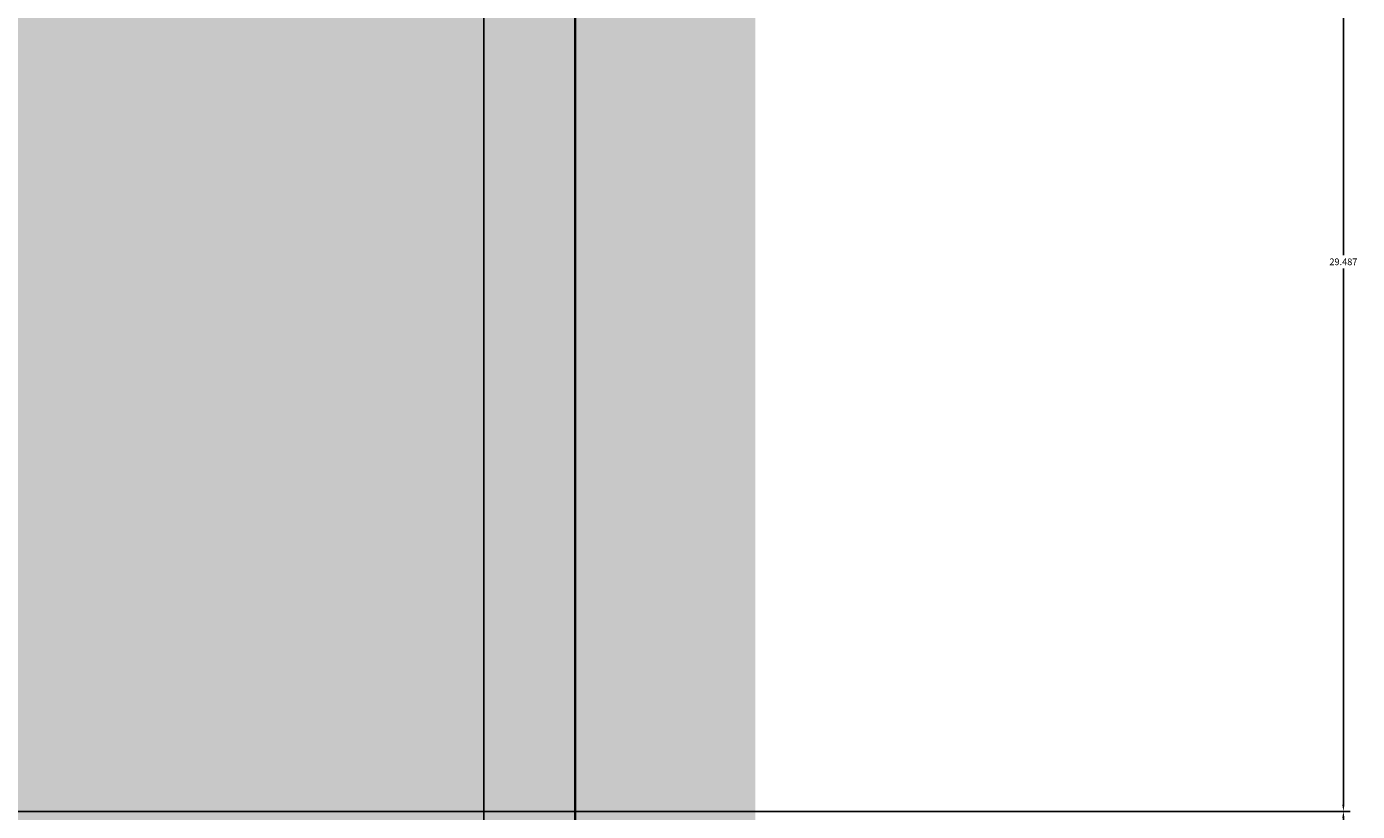
# Model space of a CAD drawing. Units: feet. Extents: x 2695 to 2912, y 795 to 1139.
# Tile 77 of 83: x 2876 to 2912, y 1021 to 1042. Entities that reach past the tile are written whole.
import ezdxf

# ---------------------------------------------------------------- set-up
doc = ezdxf.new("R2010")
doc.units = ezdxf.units.FT
for name, color, linetype, lineweight in [('A-ANNO-DIMS', 2, 'Continuous', 18), ('A-ELEV', 7, 'Continuous', 35), ('A-ELEV-PATT', 252, 'Continuous', 13)]:
    doc.layers.add(name, color=color, linetype=linetype, lineweight=lineweight)
doc.styles.get("Standard").update_dxf_attribs({"font": 'arial.ttf'})
doc.dimstyles.get("Standard").update_dxf_attribs({"dimtxt": 0.18, "dimasz": 0.18, "dimexe": 0.18, "dimexo": 0.0625, "dimgap": 0.09, "dimtad": 0, "dimtih": 1, "dimtoh": 1, "dimdec": 1, "dimzin": 0, "dimdsep": 46, "dimlunit": 3, "dimtxsty": 'Standard', "dimcen": 0.09, "dimadec": 0, "dimazin": 0, "dimtfac": 1, "dimtdec": 1, "dimtofl": 0, "dimtmove": 0, "dimatfit": 3, "dimfxl": 1, "dimtolj": 1, "dimtzin": 0, "dimarcsym": 0})

# ---------------------------------------------------------------- blocks, each defined once
blk = doc.blocks.new('*D11')
at = {"layer": 'A-ANNO-DIMS', "color": 0, "lineweight": -2, "transparency": 16777216}
for p, q in [((2843.575, 1020.886), (2843.575, 1138.886)), ((2843.755, 1138.706), (2869.128, 1138.706)), ((2895.289, 1138.706), (2869.916, 1138.706)), ((2895.469, 1107.898), (2895.469, 1138.886))]:
    blk.add_line(p, q, dxfattribs=at)
at = {"layer": 'A-ANNO-DIMS', "color": 0, "transparency": 16777216}
for points in [[(2843.755, 1138.736), (2843.755, 1138.676), (2843.575, 1138.706)], [(2895.289, 1138.736), (2895.289, 1138.676), (2895.469, 1138.706)]]:
    blk.add_solid(points, dxfattribs=at)
at = {"layer": 'Defpoints', "color": 0, "transparency": 16777216}
for p in [(2895.469, 1138.706), (2895.469, 1107.835), (2843.575, 1020.824)]:
    blk.add_point(p, dxfattribs=at)
at = {"layer": 'A-ANNO-DIMS', "color": 0, "transparency": 16777216, "insert": (2869.522, 1138.706), "char_height": 0.18, "attachment_point": 5}
blk.add_mtext('\\A1;51.89', dxfattribs=at)
blk = doc.blocks.new('*D17')
at = {"layer": 'A-ANNO-DIMS', "color": 0, "lineweight": -2, "transparency": 16777216}
for p, q in [((2843.637, 1020.824), (2911.424, 1020.824)), ((2911.244, 1020.644), (2911.244, 979.059)), ((2911.244, 937.111), (2911.244, 978.695)), ((2890.699, 936.931), (2911.424, 936.931))]:
    blk.add_line(p, q, dxfattribs=at)
at = {"layer": 'A-ANNO-DIMS', "color": 0, "transparency": 16777216}
for points in [[(2911.214, 1020.644), (2911.274, 1020.644), (2911.244, 1020.824)], [(2911.214, 937.111), (2911.274, 937.111), (2911.244, 936.931)]]:
    blk.add_solid(points, dxfattribs=at)
at = {"layer": 'Defpoints', "color": 0, "transparency": 16777216}
for p in [(2843.575, 1020.824), (2911.244, 1020.824), (2890.636, 936.931)]:
    blk.add_point(p, dxfattribs=at)
at = {"layer": 'A-ANNO-DIMS', "color": 0, "transparency": 16777216, "insert": (2911.244, 978.877), "char_height": 0.18, "attachment_point": 5}
blk.add_mtext('\\A1;83.9', dxfattribs=at)
blk = doc.blocks.new('*D18')
at = {"layer": 'A-ANNO-DIMS', "color": 0, "lineweight": -2, "transparency": 16777216}
for p, q in [((2890.699, 1050.311), (2911.424, 1050.311)), ((2911.244, 1050.131), (2911.244, 1035.749)), ((2911.244, 1021.004), (2911.244, 1035.385)), ((2843.637, 1020.824), (2911.424, 1020.824))]:
    blk.add_line(p, q, dxfattribs=at)
at = {"layer": 'A-ANNO-DIMS', "color": 0, "transparency": 16777216}
for points in [[(2911.214, 1050.131), (2911.274, 1050.131), (2911.244, 1050.311)], [(2911.214, 1021.004), (2911.274, 1021.004), (2911.244, 1020.824)]]:
    blk.add_solid(points, dxfattribs=at)
at = {"layer": 'Defpoints', "color": 0, "transparency": 16777216}
for p in [(2890.636, 1050.311), (2911.244, 1050.311), (2843.575, 1020.824)]:
    blk.add_point(p, dxfattribs=at)
at = {"layer": 'A-ANNO-DIMS', "color": 0, "transparency": 16777216, "insert": (2911.244, 1035.567), "char_height": 0.18, "attachment_point": 5}
blk.add_mtext('\\A1;29.487', dxfattribs=at)
blk = doc.blocks.new('*D50')
at = {"layer": 'A-ANNO-DIMS', "color": 0, "lineweight": -2, "transparency": 16777216}
for p, q in [((2810.041, 972.03), (2810.041, 1138.886)), ((2810.221, 1138.706), (2848.721, 1138.706)), ((2888.008, 1138.706), (2849.508, 1138.706)), ((2888.188, 972.03), (2888.188, 1138.886))]:
    blk.add_line(p, q, dxfattribs=at)
at = {"layer": 'A-ANNO-DIMS', "color": 0, "transparency": 16777216}
for points in [[(2810.221, 1138.736), (2810.221, 1138.676), (2810.041, 1138.706)], [(2888.008, 1138.736), (2888.008, 1138.676), (2888.188, 1138.706)]]:
    blk.add_solid(points, dxfattribs=at)
at = {"layer": 'Defpoints', "color": 0, "transparency": 16777216}
for p in [(2888.188, 1138.706), (2810.041, 971.967), (2888.188, 971.967)]:
    blk.add_point(p, dxfattribs=at)
at = {"layer": 'A-ANNO-DIMS', "color": 0, "transparency": 16777216, "insert": (2849.114, 1138.706), "char_height": 0.18, "attachment_point": 5}
blk.add_mtext('\\A1;78.15', dxfattribs=at)
blk = doc.blocks.new('*D51')
at = {"layer": 'A-ANNO-DIMS', "color": 0, "lineweight": -2, "transparency": 16777216}
for p, q in [((2888.188, 972.03), (2888.188, 1138.886)), ((2888.368, 1138.706), (2889.017, 1138.706)), ((2890.456, 1138.706), (2889.808, 1138.706)), ((2890.636, 972.03), (2890.636, 1138.886))]:
    blk.add_line(p, q, dxfattribs=at)
at = {"layer": 'A-ANNO-DIMS', "color": 0, "transparency": 16777216}
for points in [[(2888.368, 1138.736), (2888.368, 1138.676), (2888.188, 1138.706)], [(2890.456, 1138.736), (2890.456, 1138.676), (2890.636, 1138.706)]]:
    blk.add_solid(points, dxfattribs=at)
at = {"layer": 'Defpoints', "color": 0, "transparency": 16777216}
for p in [(2890.636, 1138.706), (2888.188, 971.967), (2890.636, 971.967)]:
    blk.add_point(p, dxfattribs=at)
at = {"layer": 'A-ANNO-DIMS', "color": 0, "transparency": 16777216, "insert": (2889.412, 1138.706), "char_height": 0.18, "attachment_point": 5}
blk.add_mtext('\\A1;2.448', dxfattribs=at)

msp = doc.modelspace()

# ---------------------------------------------------------------- hatches: boundary and pattern name
at = {"layer": 'A-ELEV-PATT'}
h = msp.add_hatch(color=256, dxfattribs=at)
h.set_gradient(color1=(147, 149, 152), color2=(147, 149, 152), tint=1)
h.paths.add_polyline_path([(2770.6361, 1118.4096), (2710.6361, 1118.4096), (2710.6361, 1062.9306), (2770.6361, 1062.9306)])
h.paths.add_polyline_path([(2890.6361, 1103.3378), (2770.6361, 1103.3378), (2770.6361, 1062.9306), (2890.6361, 1062.9306)])
h.paths.add_polyline_path([(2730.7081, 1048.1052), (2755.1125, 1048.1052), (2755.1125, 936.9306), (2770.6361, 936.9306), (2770.6361, 1050.3105), (2715.8852, 1050.3105), (2715.8852, 936.9306), (2730.7081, 936.9306)])
h.paths.add_polyline_path([(2890.6361, 1050.3105), (2770.6361, 1050.3105), (2770.6361, 971.9673), (2778.0341, 971.9673), (2778.0341, 1020.8235), (2843.575, 1020.8235), (2843.575, 971.9673), (2890.6361, 971.9673)])
h.paths.add_polyline_path([(2888.1882, 970.7156), (2843.575, 970.7156), (2843.575, 964.8267), (2888.1882, 964.8267)])
h.paths.add_polyline_path([(2888.1882, 964.1328), (2843.575, 964.1328), (2843.575, 956.614), (2888.1882, 956.614)])
h.paths.add_polyline_path([(2888.1882, 955.9202), (2843.575, 955.9202), (2843.575, 949.2892), (2888.1882, 949.2892)])
h.paths.add_polyline_path([(2888.1882, 948.5954), (2843.575, 948.5954), (2843.575, 941.3507), (2888.1882, 941.3507)])
h.paths.add_polyline_path([(2888.1882, 940.6569), (2843.575, 940.6569), (2843.575, 936.9306), (2888.1882, 936.9306)])
h.paths.add_polyline_path([(2890.6361, 970.7156), (2888.9368, 970.7156), (2888.9368, 964.8267), (2890.6361, 964.8267)])
h.paths.add_polyline_path([(2890.6361, 964.1328), (2888.9368, 964.1328), (2888.9368, 956.614), (2890.6361, 956.614)])
h.paths.add_polyline_path([(2890.6361, 955.9202), (2888.9368, 955.9202), (2888.9368, 949.2892), (2890.6361, 949.2892)])
h.paths.add_polyline_path([(2890.6361, 940.6569), (2888.9368, 940.6569), (2888.9368, 936.9306), (2890.6361, 936.9306)])
h.paths.add_polyline_path([(2890.6361, 948.5954), (2888.9368, 948.5954), (2888.9368, 941.3507), (2890.6361, 941.3507)])
h.paths.add_polyline_path([(2772.5216, 970.7156), (2770.6361, 970.7156), (2770.6361, 964.8267), (2772.5216, 964.8267)])
h.paths.add_polyline_path([(2772.5216, 964.1328), (2770.6361, 964.1328), (2770.6361, 956.614), (2772.5216, 956.614)])
h.paths.add_polyline_path([(2772.5216, 955.9202), (2770.6361, 955.9202), (2770.6361, 949.2892), (2772.5216, 949.2892)])
h.paths.add_polyline_path([(2772.5216, 948.5954), (2770.6361, 948.5954), (2770.6361, 941.3507), (2772.5216, 941.3507)])
h.paths.add_polyline_path([(2772.5216, 940.6569), (2770.6361, 940.6569), (2770.6361, 936.9306), (2772.5216, 936.9306)])
h.paths.add_polyline_path([(2778.0341, 940.6569), (2773.2702, 940.6569), (2773.2702, 936.9306), (2778.0341, 936.9306)])
h.paths.add_polyline_path([(2778.0341, 970.7156), (2773.2702, 970.7156), (2773.2702, 964.8267), (2778.0341, 964.8267)])
h.paths.add_polyline_path([(2778.0341, 964.1328), (2773.2702, 964.1328), (2773.2702, 956.614), (2778.0341, 956.614)])
h.paths.add_polyline_path([(2778.0341, 955.9202), (2773.2702, 955.9202), (2773.2702, 949.2892), (2778.0341, 949.2892)])
h.paths.add_polyline_path([(2778.0341, 948.5954), (2773.2702, 948.5954), (2773.2702, 941.3507), (2778.0341, 941.3507)])
h.paths.add_polyline_path([(2810.0407, 940.6569), (2780.0341, 940.6569), (2780.0341, 936.9306), (2810.0407, 936.9306)])
h.paths.add_polyline_path([(2890.6361, 924.3105), (2770.6361, 924.3105), (2770.6361, 810.9306), (2773.5029, 810.9306), (2773.5029, 905.5143), (2805.9398, 905.5143), (2838.3767, 905.5143), (2838.3767, 810.9306), (2890.6361, 810.9306)])
h = msp.add_hatch(color=256, dxfattribs=at)
h.set_gradient(color1=(255, 255, 255), tint=1)
h.paths.add_polyline_path([(2895.4694, 1107.8588), (2890.6361, 1107.8588), (2890.6361, 810.9306), (2895.4694, 810.9306)])
h = msp.add_hatch(color=256, dxfattribs=at)
h.set_gradient(color1=(255, 255, 255), tint=1)
h.paths.add_polyline_path([(2890.6361, 1050.3105), (2881.9484, 1050.3105), (2881.9484, 971.9673), (2890.6361, 971.9673)])
h.paths.add_polyline_path([(2888.1882, 970.7156), (2881.9484, 970.7156), (2881.9484, 964.8267), (2888.1882, 964.8267)])
h.paths.add_polyline_path([(2890.6361, 970.7156), (2888.9368, 970.7156), (2888.9368, 964.8267), (2890.6361, 964.8267)])
h.paths.add_polyline_path([(2888.1882, 964.1328), (2881.9484, 964.1328), (2881.9484, 956.614), (2888.1882, 956.614)])
h.paths.add_polyline_path([(2890.6361, 964.1328), (2888.9368, 964.1328), (2888.9368, 956.614), (2890.6361, 956.614)])
h.paths.add_polyline_path([(2888.1882, 955.9202), (2881.9484, 955.9202), (2881.9484, 949.2892), (2888.1882, 949.2892)])
h.paths.add_polyline_path([(2890.6361, 955.9202), (2888.9368, 955.9202), (2888.9368, 949.2892), (2890.6361, 949.2892)])
h.paths.add_polyline_path([(2888.1882, 948.5954), (2881.9484, 948.5954), (2881.9484, 941.3507), (2888.1882, 941.3507)])
h.paths.add_polyline_path([(2890.6361, 948.5954), (2888.9368, 948.5954), (2888.9368, 941.3507), (2890.6361, 941.3507)])
h.paths.add_polyline_path([(2888.1882, 940.6569), (2881.9484, 940.6569), (2881.9484, 936.9306), (2888.1882, 936.9306)])

# ---------------------------------------------------------------- linework, layer by layer
at = {"layer": 'A-ELEV'}
for p, q in [((2890.6361, 810.9306), (2890.6361, 1107.8588)), ((2890.6361, 1062.9306), (2890.6361, 810.9306))]:
    msp.add_line(p, q, dxfattribs=at)

# ---------------------------------------------------------------- dimensions: what is measured, and where the dimension line sits
at = {"layer": 'A-ANNO-DIMS'}
for base, p1, p2, override, picture, middle in [((2888.1882, 1138.7056), (2810.0407, 971.9673), (2888.1882, 971.9673), {"dimdec": 2, "dimlfac": 1, "dimrnd": 0, "dimzin": 0, "dimdsep": 46, "dimlunit": 2}, '*D50', (2849.1144, 1138.7056)), ((2895.4694, 1138.7056), (2843.575, 1020.8235), (2895.4694, 1107.8352), {"dimdec": 2, "dimlfac": 1, "dimrnd": 0, "dimzin": 0, "dimdsep": 46, "dimlunit": 2}, '*D11', (2869.5222, 1138.7056)), ((2890.6361, 1138.7056), (2888.1882, 971.9673), (2890.6361, 971.9673), {"dimdec": 3, "dimlfac": 1, "dimrnd": 0, "dimzin": 0, "dimdsep": 46, "dimlunit": 2}, '*D51', (2889.4121, 1138.7056))]:
    dim = msp.add_linear_dim(base=base, p1=p1, p2=p2, dimstyle='Standard', override=override, dxfattribs=at)
    dim.commit()
    dim.dimension.update_dxf_attribs({"geometry": picture, "text_midpoint": middle})
for base, p1, p2, override, picture, middle in [((2911.2444, 1050.3105), (2843.575, 1020.8235), (2890.6361, 1050.3105), {"dimdec": 3, "dimlfac": 1, "dimrnd": 0, "dimzin": 0, "dimdsep": 46, "dimlunit": 2}, '*D18', (2911.2444, 1035.567)), ((2911.2444, 1020.8235), (2890.6361, 936.9306), (2843.575, 1020.8235), {"dimdec": 1, "dimlfac": 1, "dimrnd": 0, "dimzin": 0, "dimdsep": 46, "dimlunit": 2}, '*D17', (2911.2444, 978.877))]:
    dim = msp.add_linear_dim(base=base, p1=p1, p2=p2, angle=90, dimstyle='Standard', override=override, dxfattribs=at)
    dim.commit()
    dim.dimension.update_dxf_attribs({"geometry": picture, "text_midpoint": middle})

doc.saveas('drawing.dxf')
